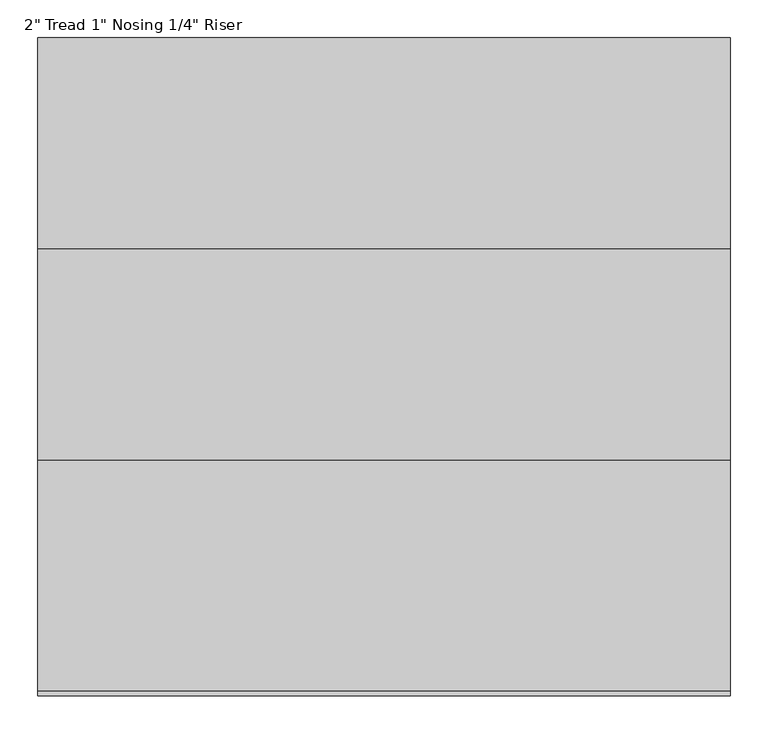
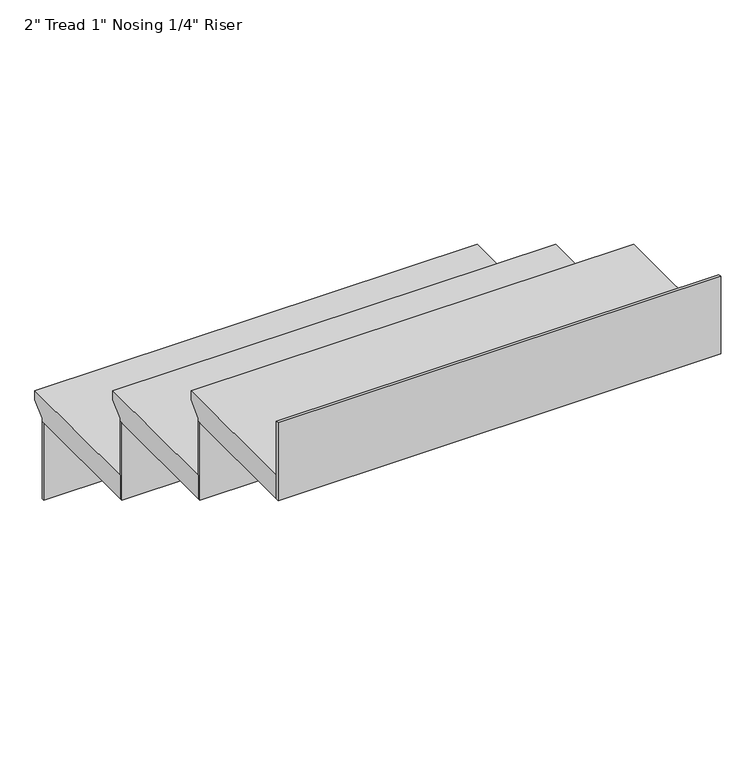
"""IFC4 building model written with IfcOpenShell, lengths in millimetres: stair flight geometry."""

from ifc_helpers import new_model, si_unit, frame, origin, place, context, project, spatial, polyline, outline, extrude, source, transform, mapped, element, save


def stair_flight_c52ec63c(model_context):
    return source(origin(), model_context, "Body", "SweptSolid", [
        extrude(outline(polyline([(-19826.9851539, 36918.6172466), (-19522.1851539, 36918.6172466), (-19522.1851539, 36899.5672466), (-19547.5851539, 36874.1672466), (-19547.5851539, 36867.8172466), (-19826.9851539, 36867.8172466), (-19826.9851539, 36918.6172466)])), frame((-2296.6415084, 0.0, 0.0), z_axis=(1.0, 0.0, 0.0), x_axis=(0.0, 1.0, 0.0)), (0.0, 0.0, 1.0), 914.4),
        extrude(outline(polyline([(-2296.6415084, -19553.9351539), (-2296.6415084, -19547.5851539), (-1382.2415084, -19547.5851539), (-1382.2415084, -19553.9351539), (-2296.6415084, -19553.9351539)])), frame((0.0, 0.0, 36698.4839133), z_axis=(0.0, 0.0, 1.0), x_axis=(1.0, 0.0, 0.0)), (0.0, 0.0, 1.0), 169.3333333),
        extrude(outline(polyline([(-2296.6415084, -19833.3351539), (-2296.6415084, -19826.9851539), (-1382.2415084, -19826.9851539), (-1382.2415084, -19833.3351539), (-2296.6415084, -19833.3351539)])), frame((0.0, 0.0, 36867.8172466), z_axis=(0.0, 0.0, 1.0), x_axis=(1.0, 0.0, 0.0)), (0.0, 0.0, 1.0), 169.3333333),
        extrude(outline(polyline([(-20106.3851539, 37087.9505799), (-19801.5851539, 37087.9505799), (-19801.5851539, 37068.9005799), (-19826.9851539, 37043.5005799), (-19826.9851539, 37037.1505799), (-20106.3851539, 37037.1505799), (-20106.3851539, 37087.9505799)])), frame((-2296.6415084, 0.0, 0.0), z_axis=(1.0, 0.0, 0.0), x_axis=(0.0, 1.0, 0.0)), (0.0, 0.0, 1.0), 914.4),
        extrude(outline(polyline([(-2296.6415084, -20112.7351539), (-2296.6415084, -20106.3851539), (-1382.2415084, -20106.3851539), (-1382.2415084, -20112.7351539), (-2296.6415084, -20112.7351539)])), frame((0.0, 0.0, 37037.1505799), z_axis=(0.0, 0.0, 1.0), x_axis=(1.0, 0.0, 0.0)), (0.0, 0.0, 1.0), 169.3333333),
        extrude(outline(polyline([(-2296.6415084, -20392.1351539), (-2296.6415084, -20385.7851539), (-1382.2415084, -20385.7851539), (-1382.2415084, -20392.1351539), (-2296.6415084, -20392.1351539)])), frame((0.0, 0.0, 37206.4839133), z_axis=(0.0, 0.0, 1.0), x_axis=(1.0, 0.0, 0.0)), (0.0, 0.0, 1.0), 169.3333333),
        extrude(outline(polyline([(-20385.7851539, 37257.2839133), (-20080.9851539, 37257.2839133), (-20080.9851539, 37238.2339133), (-20106.3851539, 37212.8339133), (-20106.3851539, 37206.4839133), (-20385.7851539, 37206.4839133), (-20385.7851539, 37257.2839133)])), frame((-2296.6415084, 0.0, 0.0), z_axis=(1.0, 0.0, 0.0), x_axis=(0.0, 1.0, 0.0)), (0.0, 0.0, 1.0), 914.4),
    ])


if __name__ == "__main__":
    model = new_model("IFC4")
    model_context = context("Model", 3, world=origin())
    ifc_project = project(units=[si_unit("LENGTHUNIT", "METRE", prefix="MILLI")], contexts=[model_context])
    site = spatial("IfcSite", under=ifc_project)
    building = spatial("IfcBuilding", under=site)
    placement = place(None, origin())
    stair_flight_shape = stair_flight_c52ec63c(model_context)
    element("IfcStairFlight", 1, ObjectType="2\" Tread 1\" Nosing 1/4\" Riser", at=placement, inside=building, context=model_context, shape_type="MappedRepresentation", body=[
        mapped(stair_flight_shape, transform((0.0, 0.0, 0.0), x_axis=(1.0, 0.0, 0.0), y_axis=(0.0, 1.0, 0.0), z_axis=(0.0, 0.0, 1.0))),
    ])
    save(model, "model.ifc")
